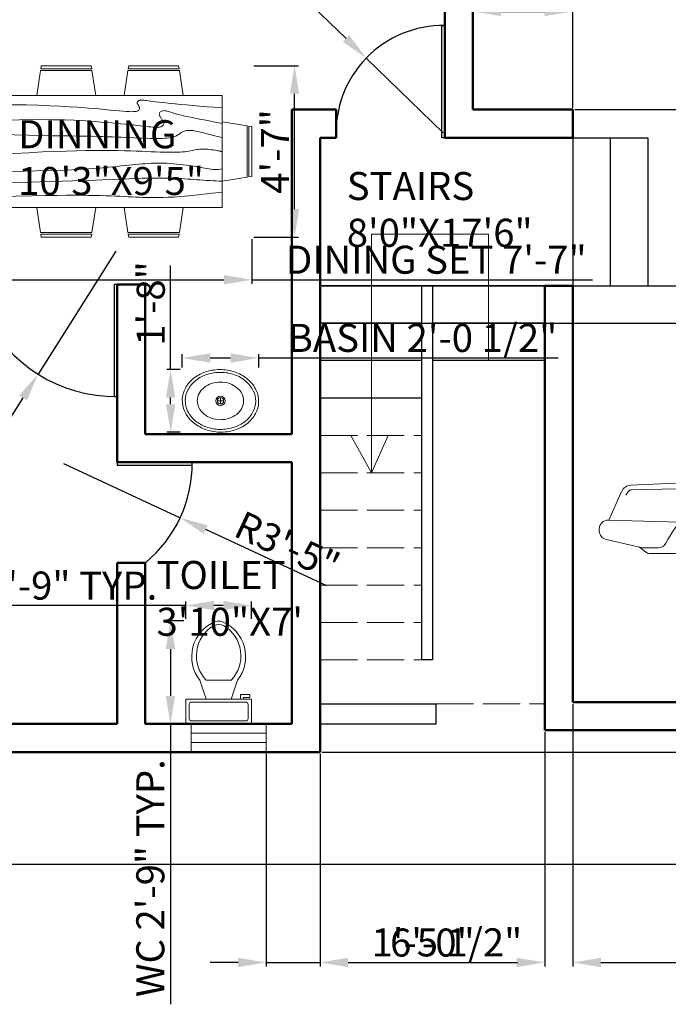
# Model space of a CAD drawing. Units: inches. Extents: x 2059616 to 2060276, y 889994 to 890582.
# Tile 2 of 4: x 2059830 to 2060037, y 890038 to 890354. Entities that reach past the tile are written whole.
import ezdxf

# ---------------------------------------------------------------- set-up
doc = ezdxf.new("R2010")
doc.units = ezdxf.units.IN
doc.linetypes.add('ACAD_ISO02W100', pattern=[15, 12, -3])
for name, color, linetype, lineweight in [('A-ANNO-DIMS', 2, 'Continuous', 18), ('A-ANNO-SYMB', 7, 'Continuous', 18), ('A-AREA-IDEN', 7, 'Continuous', 25), ('A-DOOR', 3, 'Continuous', 25), ('A-FLOR-FIXT', 9, 'Continuous', 18), ('A-FLOR-STRS', 7, 'Continuous', 25), ('A-FLOR-STRS-HIDN', 8, 'ACAD_ISO02W100', 18), ('A-FURN', 8, 'Continuous', 18), ('A-GLAZ', 4, 'Continuous', 18), ('A-SITE-VEHC', 8, 'Continuous', 18), ('A-WALL', 7, 'Continuous', 50), ('C-PROP', 7, 'Continuous', 25)]:
    doc.layers.add(name, color=color, linetype=linetype, lineweight=lineweight)
doc.styles.get("Standard").update_dxf_attribs({"font": 'arial.ttf'})
doc.dimstyles.new('ISO-25', dxfattribs={"dimtxt": 9, "dimasz": 9, "dimexe": 1.25, "dimexo": 0.625, "dimtad": 1, "dimdec": 1, "dimrnd": 9, "dimlunit": 3, "dimtxsty": 'Standard', "dimcen": 2.5, "dimadec": 0, "dimazin": 0, "dimtfac": 1, "dimtdec": 1, "dimtmove": 0, "dimatfit": 3, "dimfxl": 1, "dimarcsym": 0})

# ---------------------------------------------------------------- blocks, each defined once
blk = doc.blocks.new('Car - sedan  side')
for p, q in [((-139.53, 35.99), (-129.64, 47.91)), ((-128.57, 32.64), (-121.22, 48.02)), ((-77.81, 49.34), (-126.58, 49.34)), ((-74.7, 48.02), (-121.22, 48.02)), ((-120.32, 34.67), (-115.67, 48.02)), ((-115.4, 34.67), (-111.74, 48.02)), ((-94.41, 34.67), (-97.73, 48.02)), ((-93.72, 34.67), (-97.04, 48.02)), ((-93.03, 34.67), (-96.34, 48.02)), ((-60.02, 34.65), (-76.07, 48.02)), ((-56.87, 35.13), (-75.48, 48.59)), ((-58.54, 34.93), (-74.99, 48.02)), ((-97.55, 47.3), (-111.94, 47.3)), ((-76.26, 47.3), (-96.16, 47.3)), ((-61.08, 34.66), (-76.26, 47.3)), ((-60.02, 34.65), (-58.54, 34.93)), ((-57.21, 35.38), (-58.54, 34.93)), ((-164.57, 31.6), (-165.48, 30.35)), ((-140.23, 34.67), (-163.88, 33.56)), ((-62.28, 34.67), (-140.23, 34.67)), ((-130.39, 24.63), (-128.57, 32.64)), ((-93.72, 19.62), (-93.72, 34.67)), ((-62.28, 34.67), (-60.02, 34.65)), ((-57.97, 31.61), (-60.02, 34.65)), ((-57.97, 19.62), (-57.97, 31.61)), ((-54.93, 34.4), (-8.75, 29.8)), ((-170.93, 22.32), (-166.81, 31.56)), ((-4.21, 24.18), (-5.42, 27.27)), ((-148.26, 21.7), (-171.11, 22.33)), ((-128.78, 24.63), (-144.79, 24.63)), ((-36.97, 24.38), (-34.94, 24.38)), ((-174, 19.51), (-174, 18.91)), ((-47.2, 19.62), (-125.23, 19.62)), ((-93.72, 12.14), (-93.72, 19.62)), ((-57.97, 12.14), (-57.97, 19.62)), ((0, 19.62), (-24.7, 19.62)), ((-160.12, 13.48), (-171.81, 16.16)), ((-159.22, 12.14), (-161.08, 13.7)), ((-155.01, 13.48), (-160.12, 13.48)), ((-51.4, 9.89), (-49.69, 15.14)), ((-4.23, 13.19), (-20.72, 13.19)), ((-9.5, 13.19), (-14.1, 10.2)), ((-3.22, 13.59), (-1.77, 14.97)), ((-147.03, 11.6), (-157.73, 11.6)), ((-50.67, 12.14), (-123.32, 12.14)), ((-94.21, 9.03), (-94.21, 12.14)), ((-58.39, 9.03), (-58.39, 12.14)), ((-20.36, 11.06), (-24.06, 9.44)), ((-18.83, 10.42), (-19.11, 10.76)), ((-14.68, 10.03), (-18.01, 10.03)), ((-120.62, 9.03), (-125.23, 9.03)), ((-45.76, 9.03), (-120.62, 9.03))]:
    blk.add_line(p, q)
at = {"const_width": 5.49}
for points in [[(-127.8, 11, -1), (-144.3, 11, -1)], [(-26.69, 11, -1), (-43.19, 11, -1)]]:
    blk.add_lwpolyline(points, format="xyb", close=True, dxfattribs=at)
for centre, radius in [((-136.05, 11), 11), ((-34.94, 11), 11), ((-136.05, 11), 5.51), ((-34.94, 11), 5.51)]:
    blk.add_circle(centre, radius)
for centre, radius, start, end in [((-126.58, 45.38), 3.97, 90, 140.3029), ((-77.81, 45.38), 3.97, 54.135, 90), ((-142.58, 38.53), 3.97, 272.6827, 320.3029), ((-54.54, 38.35), 3.97, 234.135, 264.3123), ((-163.72, 30.18), 3.38, 92.6827, 155.9736), ((-163.62, 30.91), 1.17, 91.491, 143.9553), ((-118.51, -1702.12), 1734.79, 86.34698, 91.49105), ((-9.15, 25.82), 4, 21.3107, 84.3123), ((-171.18, 19.51), 2.82, 88.4193, 180), ((-118.09, -2.78), 38.85, 136.3964, 152.9097), ((-144.79, 22.64), 1.98, 90, 136.3964), ((-128.78, 22.64), 1.98, 28.1371, 90), ((-157.14, 7.48), 34.14, 6.5135, 28.1371), ((-36.97, 11), 13.38, 90, 161.9732), ((-34.94, 11), 13.38, 13.5864, 90), ((0.9, 26.18), 5.49, 201.3107, 247.7048), ((-1.92, 19.3), 1.94, 325.3744, 67.7048), ((-171.18, 18.91), 2.82, 180, 257.0905), ((-3.82, 17.12), 2.96, 313.7173, 352.3839), ((2.46, 16.28), 3.37, 145.3744, 172.3839), ((-155.01, 16.1), 2.62, 270, 332.9097), ((-20.72, 14.43), 1.24, 193.5864, 270), ((-4.23, 14.65), 1.46, 270, 313.7173), ((-157.73, 13.93), 2.32, 230.1291, 270), ((-120.62, 11.65), 2.62, 186.5135, 270), ((-52.58, 10.27), 1.24, 270, 341.9732), ((-19.93, 10.09), 1.06, 39.301, 113.7159), ((-18.01, 11.09), 1.06, 219.301, 270), ((-14.68, 11.09), 1.06, 270, 303.047)]:
    blk.add_arc(centre, radius, start, end)
blk = doc.blocks.new('Sink - Oval top')
for p, q in [((-1, 0), (1, 0)), ((0, 1), (0, -1))]:
    blk.add_line(p, q)
for points in [[(-12.23, 0.39, 0.117634), (-11.46, -3.36, 0.104469), (-8.88, -6.8, 0.090016), (-5.08, -9.07, 0.08192), (-0.32, -10.02, 0.08192), (4.49, -9.38, 0.090016), (8.42, -7.36, 0.104469), (11.22, -4.09, 0.117634), (12.23, -0.39, 0.117634), (11.46, 3.36, 0.104469), (8.88, 6.8, 0.090016), (5.08, 9.07, 0.08192), (0.32, 10.02, 0.08192), (-4.49, 9.38, 0.090016), (-8.42, 7.36, 0.104469), (-11.22, 4.09, 0.117634)], [(-11.29, 0.16, 0.118622), (-10.52, -3.25, 0.104678), (-8.07, -6.36, 0.089562), (-4.54, -8.37, 0.081185), (-0.13, -9.15, 0.081185), (4.3, -8.49, 0.089562), (7.89, -6.58, 0.104678), (10.42, -3.55, 0.118622), (11.29, -0.16, 0.118622), (10.52, 3.25, 0.104678), (8.07, 6.36, 0.089562), (4.54, 8.37, 0.081185), (0.13, 9.15, 0.081185), (-4.3, 8.49, 0.089562), (-7.89, 6.58, 0.104678), (-10.42, 3.55, 0.118622)], [(-7.42, 0.08, 0.118283), (-6.91, -2.17, 0.104607), (-5.29, -4.21, 0.089718), (-2.97, -5.53, 0.081436), (-0.07, -6.04, 0.081436), (2.84, -5.59, 0.089718), (5.2, -4.33, 0.104607), (6.86, -2.32, 0.118283), (7.42, -0.08, 0.118283), (6.91, 2.17, 0.104607), (5.29, 4.21, 0.089718), (2.97, 5.53, 0.081436), (0.07, 6.04, 0.081436), (-2.84, 5.59, 0.089718), (-5.2, 4.33, 0.104607), (-6.86, 2.32, 0.118283)]]:
    blk.add_lwpolyline(points, format="xyb", close=True)
for radius in [1.5, 1]:
    blk.add_circle((0, 0), radius)
blk = doc.blocks.new('Toilet - top')
for p, q in [((9.5, -6), (9.5, -2)), ((-10, -8.5), (-8, -8.5)), ((-10, -9.5), (-10, -8.5)), ((-8, -8.5), (-8, -8)), ((-7, -8), (-7, -9.5)), ((-4, -8), (-6, -14)), ((4, -8), (6, -14)), ((-7, -9.5), (-10, -9.5)), ((4, -14), (-4, -14))]:
    blk.add_line(p, q)
blk.add_lwpolyline([(10.5, -8), (10.5, 0), (-10.5, 0), (-10.5, -8)], close=True)
for points in [[(-9.5, -2), (-9.5, -6)], [(8.5, -1), (-8.5, -1)], [(-8.5, -7), (8.5, -7)]]:
    blk.add_lwpolyline(points)
for centre, radius, start, end in [((-8.62, -1.88), 0.884, 81.8699, 188.1301), ((8.62, -1.88), 0.884, 351.8699, 98.1301), ((-8.62, -6.12), 0.884, 171.8699, 278.1301), ((8.62, -6.12), 0.884, 261.8699, 8.1301), ((3.52, -21.58), 12.17, 141.4691, 247.9714), ((4.2, -21.82), 11.33, 136.3677, 238.9468), ((-3.52, -21.58), 12.17, 292.0284, 38.5307), ((-4.2, -21.82), 11.33, 301.053, 43.6321), ((0, -27.88), 4, 245.7318, 294.2682), ((0, -29), 4, 254.8605, 285.1395)]:
    blk.add_arc(centre, radius, start, end)
blk = doc.blocks.new('Dining Set - 36 x 72 in.')
for p, q in [((-22.2343, 26.00059), (-23.4847, 17.99762)), ((-22.2304, 26), (-5.7608, 26)), ((-22, 27.5), (-22.1562, 26.50042)), ((-5.8416, 26.5), (-22.1534, 26.5)), ((-22, 27.5), (-6, 27.5)), ((-5.8437, 26.49966), (-6, 27.5)), ((-4.5152, 17.99762), (-5.7655, 25.99926)), ((5.7657, 26.00059), (4.5153, 17.99762)), ((5.7696, 26), (22.2392, 26)), ((6, 27.5), (5.8438, 26.50042)), ((22.1584, 26.5), (5.8466, 26.5)), ((6, 27.5), (22, 27.5)), ((22.1563, 26.49966), (22, 27.5)), ((23.4848, 17.99762), (22.2345, 25.99926)), ((36, 18), (-36, 18)), ((-36, 18), (-36, -18)), ((36, -18), (36, 18)), ((-44.0006, 8.23428), (-35.9976, 9.48474)), ((44.0006, 8.23428), (35.9976, 9.48474)), ((-45.5, 8), (-44.5004, 8.15617)), ((-45.5, 8), (-45.5, -8)), ((-44.5, -8.15843), (-44.5, 8.15338)), ((-44, 8.23041), (-44, -8.23915)), ((44, 8.23041), (44, -8.23915)), ((44.5, -8.15843), (44.5, 8.15338)), ((45.5, 8), (44.5005, 8.15617)), ((45.5, 8), (45.5, -8)), ((-44.4997, -8.15631), (-45.5, -8)), ((-35.9976, -9.48476), (-43.9993, -8.2345)), ((35.9976, -9.48476), (43.9993, -8.2345)), ((44.4997, -8.15631), (45.5, -8)), ((-36, -18), (36, -18)), ((-22.2343, -26.0006), (-23.4847, -17.99762)), ((-4.5152, -17.99762), (-5.7655, -25.99928)), ((5.7657, -26.0006), (4.5153, -17.99762)), ((23.4848, -17.99762), (22.2345, -25.99928)), ((-22.2304, -26), (-5.7608, -26)), ((-22, -27.5), (-22.1562, -26.50044)), ((-5.8416, -26.5), (-22.1534, -26.5)), ((-22, -27.5), (-6, -27.5)), ((-5.8437, -26.49967), (-6, -27.5)), ((5.7696, -26), (22.2392, -26)), ((6, -27.5), (5.8438, -26.50044)), ((22.1584, -26.5), (5.8466, -26.5)), ((6, -27.5), (22, -27.5)), ((22.1563, -26.49967), (22, -27.5))]:
    blk.add_line(p, q)
for points in [[(-36, 15), (-31.1772, 14.97754), (-26.8079, 14.91406), (-22.8538, 14.81543), (-19.276, 14.6875), (-16.0362, 14.53613), (-13.0957, 14.36718), (-10.4159, 14.18652), (-7.9583, 14), (-5.6904, 13.81315), (-3.6035, 13.63021), (-1.6954, 13.45508), (0.0365, 13.29166), (1.5945, 13.14388), (2.9811, 13.01562), (4.1988, 12.9108), (5.25, 12.83333), (6.1393, 12.78613), (6.8802, 12.76823), (7.4883, 12.77767), (7.9792, 12.8125), (8.3685, 12.87077), (8.6719, 12.95052), (8.9049, 13.0498), (9.0833, 13.16666), (9.2205, 13.29899), (9.3216, 13.44401), (9.3895, 13.59879), (9.4271, 13.76041), (9.4373, 13.92594), (9.4232, 14.09245), (9.3875, 14.257), (9.3333, 14.41666), (9.2638, 14.56917), (9.1836, 14.71484), (9.0975, 14.85465), (9.0104, 14.98958), (8.9272, 15.1206), (8.8529, 15.2487), (8.7922, 15.37483), (8.75, 15.5), (8.7305, 15.62467), (8.7344, 15.74739), (8.7617, 15.86621), (8.8125, 15.97916), (8.8867, 16.08431), (8.9844, 16.17968), (9.1055, 16.26334), (9.25, 16.33333), (9.4189, 16.38802), (9.6172, 16.42708), (9.8506, 16.45052), (10.125, 16.45833), (10.4463, 16.45052), (10.8203, 16.42708), (11.2529, 16.38802), (11.75, 16.33333), (12.3184, 16.26318), (12.9694, 16.17838), (13.7151, 16.07991), (14.5677, 15.96875), (15.5395, 15.84586), (16.6426, 15.71224), (17.8893, 15.56884), (19.2917, 15.41666), (20.859, 15.25667), (22.5879, 15.08984), (24.4721, 14.91715), (26.5052, 14.73958), (28.6809, 14.5581), (30.9929, 14.3737), (33.4347, 14.18733), (36, 14)], [(-36, 10), (-28.9766, 10.14274), (-23.1725, 10.20442), (-18.4241, 10.19775), (-14.5677, 10.13541), (-11.4399, 10.03011), (-8.877, 9.89453), (-6.7154, 9.74137), (-4.7917, 9.58333), (-2.9698, 9.43082), (-1.2246, 9.28515), (0.4415, 9.14534), (2.026, 9.01041), (3.5266, 8.87939), (4.9408, 8.7513), (6.266, 8.62516), (7.5, 8.5), (8.6411, 8.37549), (9.6914, 8.2539), (10.6538, 8.13818), (11.5312, 8.03125), (12.3267, 7.93603), (13.043, 7.85547), (13.6831, 7.79248), (14.25, 7.75), (14.7471, 7.7303), (15.1797, 7.73307), (15.5537, 7.75732), (15.875, 7.80208), (16.1494, 7.86637), (16.3828, 7.94922), (16.5811, 8.04964), (16.75, 8.16666), (16.8944, 8.29915), (17.0143, 8.44531), (17.1089, 8.60319), (17.1771, 8.77083), (17.218, 8.94629), (17.2305, 9.1276), (17.2137, 9.31282), (17.1667, 9.5), (17.0895, 9.6875), (16.987, 9.875), (16.8649, 10.0625), (16.7292, 10.25), (16.5856, 10.4375), (16.4401, 10.625), (16.2985, 10.8125), (16.1667, 11), (16.05, 11.18733), (15.9518, 11.3737), (15.8752, 11.5581), (15.8229, 11.73958), (15.798, 11.91715), (15.8034, 12.08984), (15.842, 12.25667), (15.9167, 12.41666), (16.0295, 12.56836), (16.1784, 12.70833), (16.3605, 12.83268), (16.5729, 12.9375), (16.8127, 13.01888), (17.0768, 13.07291), (17.3625, 13.0957), (17.6667, 13.08333), (17.9894, 13.03312), (18.3418, 12.94726), (18.7382, 12.82918), (19.1927, 12.68229), (19.7195, 12.51001), (20.3327, 12.31575), (21.0465, 12.10294), (21.875, 11.875), (22.8357, 11.63354), (23.959, 11.37304), (25.2786, 11.08618), (26.8282, 10.76562), (28.6414, 10.40405), (30.752, 9.99414), (33.1936, 9.52856), (36, 9)], [(-36, 5.5), (-30.7157, 5.3348), (-26.069, 5.20963), (-21.9946, 5.11767), (-18.4271, 5.05208), (-15.3009, 5.00602), (-12.5508, 4.97265), (-10.1112, 4.94515), (-7.9167, 4.91666), (-5.909, 4.88167), (-4.0586, 4.83984), (-2.3429, 4.79215), (-0.7396, 4.73958), (0.7739, 4.6831), (2.22, 4.6237), (3.6213, 4.56233), (5, 4.5), (6.373, 4.43782), (7.7344, 4.3776), (9.0723, 4.32129), (10.375, 4.27083), (11.6309, 4.22819), (12.8281, 4.19531), (13.9551, 4.17415), (15, 4.16666), (15.954, 4.17448), (16.819, 4.19791), (17.6001, 4.23698), (18.3021, 4.29166), (18.9299, 4.36198), (19.4883, 4.44791), (19.9823, 4.54948), (20.4167, 4.66666), (20.7969, 4.79899), (21.1302, 4.94401), (21.4245, 5.09879), (21.6875, 5.26041), (21.9271, 5.42594), (22.1511, 5.59245), (22.3672, 5.757), (22.5834, 5.91666), (22.8065, 6.06868), (23.0404, 6.21093), (23.2879, 6.34147), (23.5521, 6.45833), (23.8358, 6.55957), (24.142, 6.64323), (24.4735, 6.70735), (24.8334, 6.75), (25.2235, 6.76969), (25.642, 6.76692), (26.0858, 6.74267), (26.5521, 6.69791), (27.0379, 6.63362), (27.5404, 6.55078), (28.0565, 6.45036), (28.5834, 6.33333), (29.1242, 6.19987), (29.7071, 6.04687), (30.3661, 5.87044), (31.1354, 5.66666), (32.0493, 5.43164), (33.142, 5.16146), (34.4475, 4.85221), (36, 4.5)], [(-36, -1), (-30.7915, -0.6591), (-26.0195, -0.38216), (-21.6519, -0.16284), (-17.6563, 0.00521), (-14.0005, 0.12833), (-10.6523, 0.21289), (-7.5796, 0.26522), (-4.75, 0.29166), (-2.134, 0.29793), (0.2878, 0.28711), (2.5317, 0.26163), (4.6146, 0.22396), (6.5529, 0.17651), (8.3633, 0.12174), (10.0623, 0.06209), (11.6667, 0), (13.1899, -0.06201), (14.6341, -0.1211), (15.9982, -0.17432), (17.2813, -0.21875), (18.4823, -0.25147), (19.6003, -0.26953), (20.6343, -0.27002), (21.5834, -0.25), (22.4481, -0.20768), (23.2357, -0.14584), (23.9549, -0.06836), (24.6146, 0.02083), (25.2235, 0.11784), (25.7904, 0.21875), (26.3241, 0.31966), (26.8334, 0.41666), (27.3265, 0.50618), (27.8099, 0.58593), (28.2894, 0.65397), (28.7709, 0.70833), (29.2601, 0.74707), (29.763, 0.76823), (30.2855, 0.76985), (30.8334, 0.75), (31.4088, 0.70784), (31.9994, 0.64713), (32.589, 0.57275), (33.1615, 0.48958), (33.7008, 0.4025), (34.1908, 0.3164), (34.6153, 0.23616), (34.9584, 0.16666), (35.2099, 0.11165), (35.3848, 0.07031), (35.504, 0.04069), (35.5886, 0.02083), (35.6594, 0.00879), (35.7377, 0.0026), (35.8442, 0.00032), (36, 0)], [(-36, -6.5), (-27.1843, -6.31267), (-20.084, -6.1263), (-14.469, -5.9419), (-10.1094, -5.76042), (-6.7752, -5.58285), (-4.2363, -5.41016), (-2.2629, -5.24333), (-0.625, -5.08334), (0.8708, -4.93099), (2.2715, -4.78646), (3.5872, -4.64974), (4.8281, -4.52084), (6.0046, -4.39974), (7.127, -4.28646), (8.2053, -4.18099), (9.25, -4.08334), (10.2705, -3.99382), (11.2734, -3.91407), (12.2647, -3.84603), (13.25, -3.79167), (14.2354, -3.75293), (15.2266, -3.73177), (16.2295, -3.73015), (17.25, -3.75), (18.2912, -3.79248), (19.3451, -3.85547), (20.4009, -3.93604), (21.4479, -4.03125), (22.4754, -4.13819), (23.4727, -4.25391), (24.4289, -4.37549), (25.3334, -4.5), (26.1785, -4.62492), (26.9694, -4.74935), (27.7145, -4.87281), (28.4219, -4.99479), (29.1, -5.11483), (29.7572, -5.23242), (30.4016, -5.34709), (31.0417, -5.45834), (31.6837, -5.56437), (32.3262, -5.65821), (32.9658, -5.73153), (33.599, -5.77604), (34.2224, -5.78345), (34.8327, -5.74545), (35.4264, -5.65373), (36, -5.5)], [(-36, -10), (-26.4022, -9.81299), (-18.4675, -9.62891), (-11.9839, -9.45069), (-6.7396, -9.28125), (-2.5226, -9.12354), (0.8789, -8.98047), (3.6769, -8.85498), (6.0833, -8.75), (8.2767, -8.66765), (10.3021, -8.60677), (12.1712, -8.56543), (13.8958, -8.54167), (15.4876, -8.53353), (16.9583, -8.53907), (18.3197, -8.55632), (19.5834, -8.58334), (20.7616, -8.61841), (21.8685, -8.66081), (22.9188, -8.71004), (23.9271, -8.76563), (24.9081, -8.82707), (25.8763, -8.89388), (26.8465, -8.96558), (27.8334, -9.04167), (28.8474, -9.12118), (29.8828, -9.20117), (30.93, -9.27824), (31.9792, -9.34896), (33.0205, -9.40991), (34.0443, -9.45768), (35.0407, -9.48885), (36, -9.5)], [(-36, -14.5), (-30.0881, -14.33513), (-25.0332, -14.21224), (-20.7312, -14.12647), (-17.0781, -14.07292), (-13.97, -14.04671), (-11.3027, -14.04297), (-8.9724, -14.05681), (-6.875, -14.08334), (-4.9224, -14.11833), (-3.0905, -14.16016), (-1.3709, -14.20785), (0.2448, -14.26042), (1.7647, -14.3169), (3.1973, -14.3763), (4.5507, -14.43767), (5.8333, -14.5), (7.0554, -14.5621), (8.235, -14.62175), (9.3922, -14.67652), (10.5469, -14.72396), (11.7192, -14.76164), (12.929, -14.78711), (14.1965, -14.79794), (15.5417, -14.79167), (16.9933, -14.76424), (18.6152, -14.70508), (20.4804, -14.60197), (22.6615, -14.44271), (25.2312, -14.21509), (28.2624, -13.9069), (31.8277, -13.50594), (36, -13)]]:
    blk.add_lwpolyline(points)
blk = doc.blocks.new('WIN-24IN')
for p, q in [((0, 24), (9, 24)), ((3, 24), (3, 0)), ((6, 24), (6, 0)), ((0, 0), (9, 0))]:
    blk.add_line(p, q)
blk = doc.blocks.new('*D24')
at = {"layer": 'A-ANNO-DIMS', "color": 0, "lineweight": -2, "transparency": 16777216}
for p, q in [((2059882.14, 890160.89), (2059876.56, 890160.89)), ((2059877.81, 890151.89), (2059877.81, 890136.85)), ((2059882.14, 890127.85), (2059876.56, 890127.85)), ((2059877.81, 890127.85), (2059877.81, 890037.93))]:
    blk.add_line(p, q, dxfattribs=at)
at = {"layer": 'A-ANNO-DIMS', "color": 0, "transparency": 16777216}
for points in [[(2059876.31, 890151.89), (2059879.31, 890151.89), (2059877.81, 890160.89)], [(2059876.31, 890136.85), (2059879.31, 890136.85), (2059877.81, 890127.85)]]:
    blk.add_solid(points, dxfattribs=at)
at = {"layer": 'Defpoints', "color": 0, "transparency": 16777216}
for p in [(2059882.76, 890160.89), (2059877.81, 890127.85), (2059882.76, 890127.85)]:
    blk.add_point(p, dxfattribs=at)
at = {"layer": 'A-ANNO-DIMS', "color": 0, "transparency": 16777216, "insert": (2059872.53, 890078.39), "char_height": 9, "attachment_point": 5, "rotation": 90}
blk.add_mtext('WC 2\'-9" TYP.', dxfattribs=at)
blk = doc.blocks.new('*D25')
at = {"layer": 'A-ANNO-DIMS', "color": 0, "lineweight": -2, "transparency": 16777216}
for p, q in [((2059882.76, 890165.85), (2059818.5, 890165.85)), ((2059882.76, 890161.52), (2059882.76, 890167.1)), ((2059894.76, 890165.85), (2059891.76, 890165.85)), ((2059903.76, 890161.52), (2059903.76, 890167.1))]:
    blk.add_line(p, q, dxfattribs=at)
at = {"layer": 'A-ANNO-DIMS', "color": 0, "transparency": 16777216}
for points in [[(2059891.76, 890167.35), (2059891.76, 890164.35), (2059882.76, 890165.85)], [(2059894.76, 890167.35), (2059894.76, 890164.35), (2059903.76, 890165.85)]]:
    blk.add_solid(points, dxfattribs=at)
at = {"layer": 'Defpoints', "color": 0, "transparency": 16777216}
for p in [(2059882.76, 890165.85), (2059882.76, 890160.89), (2059903.76, 890160.89)]:
    blk.add_point(p, dxfattribs=at)
at = {"layer": 'A-ANNO-DIMS', "color": 0, "transparency": 16777216, "insert": (2059846.13, 890171.07), "char_height": 9, "attachment_point": 5}
blk.add_mtext('1\'-9" TYP.', dxfattribs=at)
blk = doc.blocks.new('*D28')
at = {"layer": 'A-ANNO-DIMS', "color": 0, "lineweight": -2, "transparency": 16777216}
for p, q in [((2059881.56, 890242.17), (2059881.56, 890246.48)), ((2059890.56, 890245.23), (2059897.11, 890245.23)), ((2059906.11, 890242.17), (2059906.11, 890246.48)), ((2059906.11, 890245.23), (2060002.08, 890245.23))]:
    blk.add_line(p, q, dxfattribs=at)
at = {"layer": 'A-ANNO-DIMS', "color": 0, "transparency": 16777216}
for points in [[(2059890.56, 890246.73), (2059890.56, 890243.73), (2059881.56, 890245.23)], [(2059897.11, 890246.73), (2059897.11, 890243.73), (2059906.11, 890245.23)]]:
    blk.add_solid(points, dxfattribs=at)
at = {"layer": 'Defpoints', "color": 0, "transparency": 16777216}
for p in [(2059906.11, 890245.23), (2059881.56, 890241.54), (2059906.11, 890241.54)]:
    blk.add_point(p, dxfattribs=at)
at = {"layer": 'A-ANNO-DIMS', "color": 0, "transparency": 16777216, "insert": (2059958.6, 890250.51), "char_height": 9, "attachment_point": 5}
blk.add_mtext('BASIN 2\'-0 1/2"', dxfattribs=at)
blk = doc.blocks.new('*D29')
at = {"layer": 'A-ANNO-DIMS', "color": 0, "lineweight": -2, "transparency": 16777216}
for p, q in [((2059877.88, 890241.54), (2059877.88, 890274.87)), ((2059880.93, 890241.54), (2059876.63, 890241.54)), ((2059877.88, 890230.41), (2059877.88, 890232.54)), ((2059880.93, 890221.41), (2059876.63, 890221.41))]:
    blk.add_line(p, q, dxfattribs=at)
at = {"layer": 'A-ANNO-DIMS', "color": 0, "transparency": 16777216}
for points in [[(2059876.38, 890232.54), (2059879.38, 890232.54), (2059877.88, 890241.54)], [(2059876.38, 890230.41), (2059879.38, 890230.41), (2059877.88, 890221.41)]]:
    blk.add_solid(points, dxfattribs=at)
at = {"layer": 'Defpoints', "color": 0, "transparency": 16777216}
for p in [(2059877.88, 890241.54), (2059881.56, 890241.54), (2059881.56, 890221.41)]:
    blk.add_point(p, dxfattribs=at)
at = {"layer": 'A-ANNO-DIMS', "color": 0, "transparency": 16777216, "insert": (2059872.66, 890262.71), "char_height": 9, "attachment_point": 5, "rotation": 90}
blk.add_mtext('1\'-8"', dxfattribs=at)
blk = doc.blocks.new('*D36')
at = {"layer": 'A-ANNO-DIMS', "color": 0, "lineweight": -2, "transparency": 16777216}
for p, q in [((2059812.93, 890283.34), (2059812.93, 890269.07)), ((2059903.93, 890283.34), (2059903.93, 890269.07)), ((2059821.93, 890270.32), (2059894.93, 890270.32)), ((2059903.93, 890270.32), (2060013.1, 890270.32))]:
    blk.add_line(p, q, dxfattribs=at)
at = {"layer": 'A-ANNO-DIMS', "color": 0, "transparency": 16777216}
for points in [[(2059821.93, 890271.82), (2059821.93, 890268.82), (2059812.93, 890270.32)], [(2059894.93, 890271.82), (2059894.93, 890268.82), (2059903.93, 890270.32)]]:
    blk.add_solid(points, dxfattribs=at)
at = {"layer": 'Defpoints', "color": 0, "transparency": 16777216}
for p in [(2059812.93, 890283.97), (2059903.93, 890283.97), (2059903.93, 890270.32)]:
    blk.add_point(p, dxfattribs=at)
at = {"layer": 'A-ANNO-DIMS', "color": 0, "transparency": 16777216, "insert": (2059963.02, 890275.59), "char_height": 9, "attachment_point": 5}
blk.add_mtext('DINING SET 7\'-7"', dxfattribs=at)
blk = doc.blocks.new('*D37')
at = {"layer": 'A-ANNO-DIMS', "color": 0, "lineweight": -2, "transparency": 16777216}
for p, q in [((2059904.56, 890338.97), (2059918.83, 890338.97)), ((2059917.58, 890292.97), (2059917.58, 890329.97)), ((2059904.56, 890283.97), (2059918.83, 890283.97))]:
    blk.add_line(p, q, dxfattribs=at)
at = {"layer": 'A-ANNO-DIMS', "color": 0, "transparency": 16777216}
for points in [[(2059916.08, 890329.97), (2059919.08, 890329.97), (2059917.58, 890338.97)], [(2059916.08, 890292.97), (2059919.08, 890292.97), (2059917.58, 890283.97)]]:
    blk.add_solid(points, dxfattribs=at)
at = {"layer": 'Defpoints', "color": 0, "transparency": 16777216}
for p in [(2059903.93, 890338.97), (2059917.58, 890338.97), (2059903.93, 890283.97)]:
    blk.add_point(p, dxfattribs=at)
at = {"layer": 'A-ANNO-DIMS', "color": 0, "transparency": 16777216, "insert": (2059912.46, 890311.47), "char_height": 9, "attachment_point": 5, "rotation": 90}
blk.add_mtext('4\'-7"', dxfattribs=at)
blk = doc.blocks.new('*D39')
at = {"layer": 'A-ANNO-DIMS', "color": 0, "lineweight": -2, "transparency": 16777216}
for p, q in [((2060202.39, 890497.85), (2060275.51, 890497.85)), ((2060274.26, 890127.85), (2060274.26, 890488.85)), ((2059926.39, 890118.85), (2060275.51, 890118.85))]:
    blk.add_line(p, q, dxfattribs=at)
at = {"layer": 'A-ANNO-DIMS', "color": 0, "transparency": 16777216}
for points in [[(2060272.76, 890488.85), (2060275.76, 890488.85), (2060274.26, 890497.85)], [(2060272.76, 890127.85), (2060275.76, 890127.85), (2060274.26, 890118.85)]]:
    blk.add_solid(points, dxfattribs=at)
at = {"layer": 'Defpoints', "color": 0, "transparency": 16777216}
for p in [(2060201.76, 890497.85), (2060274.26, 890497.85), (2059925.76, 890118.85)]:
    blk.add_point(p, dxfattribs=at)
at = {"layer": 'A-ANNO-DIMS', "color": 0, "transparency": 16777216, "insert": (2060269.04, 890308.35), "char_height": 9, "attachment_point": 5, "rotation": 90}
blk.add_mtext('31\'-7"', dxfattribs=at)
blk = doc.blocks.new('*D52')
at = {"layer": 'A-ANNO-DIMS', "color": 0, "lineweight": -2, "transparency": 16777216}
for p, q in [((2059908.5, 890118.22), (2059908.5, 890050.1)), ((2059925.76, 890118.22), (2059925.76, 890050.1)), ((2059899.5, 890051.35), (2059890.5, 890051.35)), ((2059908.5, 890051.35), (2059925.76, 890051.35)), ((2059934.76, 890051.35), (2059989.06, 890051.35))]:
    blk.add_line(p, q, dxfattribs=at)
at = {"layer": 'A-ANNO-DIMS', "color": 0, "transparency": 16777216}
for points in [[(2059899.5, 890052.85), (2059899.5, 890049.85), (2059908.5, 890051.35)], [(2059934.76, 890052.85), (2059934.76, 890049.85), (2059925.76, 890051.35)]]:
    blk.add_solid(points, dxfattribs=at)
at = {"layer": 'Defpoints', "color": 0, "transparency": 16777216}
for p in [(2059908.5, 890118.85), (2059925.76, 890118.85), (2059925.76, 890051.35)]:
    blk.add_point(p, dxfattribs=at)
at = {"layer": 'A-ANNO-DIMS', "color": 0, "transparency": 16777216, "insert": (2059966.41, 890056.62), "char_height": 9, "attachment_point": 5}
blk.add_mtext('1\'-5 1/2"', dxfattribs=at)
blk = doc.blocks.new('*D54')
at = {"layer": 'A-ANNO-DIMS', "color": 0, "lineweight": -2, "transparency": 16777216}
for p, q in [((2059974.76, 890325.51), (2059974.76, 890357.64)), ((2060006.76, 890325.51), (2060006.76, 890357.64)), ((2059983.76, 890356.39), (2059997.76, 890356.39))]:
    blk.add_line(p, q, dxfattribs=at)
at = {"layer": 'A-ANNO-DIMS', "color": 0, "transparency": 16777216}
for points in [[(2059983.76, 890357.89), (2059983.76, 890354.89), (2059974.76, 890356.39)], [(2059997.76, 890357.89), (2059997.76, 890354.89), (2060006.76, 890356.39)]]:
    blk.add_solid(points, dxfattribs=at)
at = {"layer": 'Defpoints', "color": 0, "transparency": 16777216}
for p in [(2060006.76, 890356.39), (2059974.76, 890324.89), (2060006.76, 890324.89)]:
    blk.add_point(p, dxfattribs=at)
at = {"layer": 'A-ANNO-DIMS', "color": 0, "transparency": 16777216, "insert": (2059990.76, 890361.61), "char_height": 9, "attachment_point": 5}
blk.add_mtext('2\'-8"', dxfattribs=at)
blk = doc.blocks.new('*D55')
at = {"layer": 'A-ANNO-DIMS', "color": 0, "lineweight": -2, "transparency": 16777216}
for p, q in [((2060007.39, 890324.89), (2060275.51, 890324.89)), ((2060274.26, 890315.89), (2060274.26, 890143.85)), ((2060007.39, 890134.85), (2060275.51, 890134.85))]:
    blk.add_line(p, q, dxfattribs=at)
at = {"layer": 'A-ANNO-DIMS', "color": 0, "transparency": 16777216}
for points in [[(2060272.76, 890315.89), (2060275.76, 890315.89), (2060274.26, 890324.89)], [(2060272.76, 890143.85), (2060275.76, 890143.85), (2060274.26, 890134.85)]]:
    blk.add_solid(points, dxfattribs=at)
at = {"layer": 'Defpoints', "color": 0, "transparency": 16777216}
for p in [(2060006.76, 890324.89), (2060006.76, 890134.85), (2060274.26, 890134.85)]:
    blk.add_point(p, dxfattribs=at)
at = {"layer": 'A-ANNO-DIMS', "color": 0, "transparency": 16777216, "insert": (2060269.04, 890229.87), "char_height": 9, "attachment_point": 5, "rotation": 90}
blk.add_mtext('15\'-10"', dxfattribs=at)
blk = doc.blocks.new('*D56')
at = {"layer": 'A-ANNO-DIMS', "color": 0, "lineweight": -2, "transparency": 16777216}
for p, q in [((2060006.76, 890134.22), (2060006.76, 890050.1)), ((2060192.76, 890134.22), (2060192.76, 890050.1)), ((2060015.76, 890051.35), (2060183.76, 890051.35))]:
    blk.add_line(p, q, dxfattribs=at)
at = {"layer": 'A-ANNO-DIMS', "color": 0, "transparency": 16777216}
for points in [[(2060015.76, 890052.85), (2060015.76, 890049.85), (2060006.76, 890051.35)], [(2060183.76, 890052.85), (2060183.76, 890049.85), (2060192.76, 890051.35)]]:
    blk.add_solid(points, dxfattribs=at)
at = {"layer": 'Defpoints', "color": 0, "transparency": 16777216}
for p in [(2060006.76, 890134.85), (2060192.76, 890134.85), (2060192.76, 890051.35)]:
    blk.add_point(p, dxfattribs=at)
at = {"layer": 'A-ANNO-DIMS', "color": 0, "transparency": 16777216, "insert": (2060099.76, 890056.57), "char_height": 9, "attachment_point": 5}
blk.add_mtext('15\'-6"', dxfattribs=at)
blk = doc.blocks.new('*D57')
at = {"layer": 'A-ANNO-DIMS', "color": 0, "lineweight": -2, "transparency": 16777216}
for p, q in [((2059997.76, 890125.22), (2059997.76, 890050.1)), ((2059925.76, 890118.22), (2059925.76, 890050.1)), ((2059934.76, 890051.35), (2059988.76, 890051.35))]:
    blk.add_line(p, q, dxfattribs=at)
at = {"layer": 'A-ANNO-DIMS', "color": 0, "transparency": 16777216}
for points in [[(2059934.76, 890052.85), (2059934.76, 890049.85), (2059925.76, 890051.35)], [(2059988.76, 890052.85), (2059988.76, 890049.85), (2059997.76, 890051.35)]]:
    blk.add_solid(points, dxfattribs=at)
at = {"layer": 'Defpoints', "color": 0, "transparency": 16777216}
for p in [(2059997.76, 890125.85), (2059925.76, 890118.85), (2059997.76, 890051.35)]:
    blk.add_point(p, dxfattribs=at)
at = {"layer": 'A-ANNO-DIMS', "color": 0, "transparency": 16777216, "insert": (2059961.76, 890056.57), "char_height": 9, "attachment_point": 5}
blk.add_mtext('6\'-0"', dxfattribs=at)
blk = doc.blocks.new('*D59')
at = {"layer": 'A-ANNO-DIMS', "color": 0, "lineweight": -2, "transparency": 16777216}
for p, q in [((2060274.26, 890277.39), (2060274.26, 890310.71)), ((2059926.39, 890268.39), (2060275.51, 890268.39)), ((2060274.26, 890256.39), (2060274.26, 890268.39)), ((2059926.39, 890256.39), (2060275.51, 890256.39)), ((2060274.26, 890247.39), (2060274.26, 890238.39))]:
    blk.add_line(p, q, dxfattribs=at)
at = {"layer": 'A-ANNO-DIMS', "color": 0, "transparency": 16777216}
for points in [[(2060272.76, 890277.39), (2060275.76, 890277.39), (2060274.26, 890268.39)], [(2060272.76, 890247.39), (2060275.76, 890247.39), (2060274.26, 890256.39)]]:
    blk.add_solid(points, dxfattribs=at)
at = {"layer": 'Defpoints', "color": 0, "transparency": 16777216}
for p in [(2059925.76, 890268.39), (2060274.26, 890268.39), (2059925.76, 890256.39)]:
    blk.add_point(p, dxfattribs=at)
at = {"layer": 'A-ANNO-DIMS', "color": 0, "transparency": 16777216, "insert": (2060269.04, 890298.55), "char_height": 9, "attachment_point": 5, "rotation": 90}
blk.add_mtext('1\'-0"', dxfattribs=at)
blk = doc.blocks.new('*D60')
at = {"layer": 'A-ANNO-DIMS', "color": 0, "lineweight": -2, "transparency": 16777216}
for p, q in [((2059860.26, 890279.49), (2059835.38, 890240.04)), ((2059792.83, 890172.58), (2059830.58, 890232.42))]:
    blk.add_line(p, q, dxfattribs=at)
at = {"layer": 'A-ANNO-DIMS', "color": 0, "transparency": 16777216}
blk.add_solid([(2059829.31, 890233.22), (2059831.85, 890231.62), (2059835.38, 890240.04)], dxfattribs=at)
at = {"layer": 'Defpoints', "color": 0, "transparency": 16777216}
for p in [(2059860.26, 890279.49), (2059835.38, 890240.04)]:
    blk.add_point(p, dxfattribs=at)
at = {"layer": 'A-ANNO-DIMS', "color": 0, "transparency": 16777216, "insert": (2059804.84, 890201.51), "char_height": 9, "attachment_point": 5, "rotation": 57.7581}
blk.add_mtext('R3\'-10 1/2"', dxfattribs=at)
blk = doc.blocks.new('*D61')
at = {"layer": 'A-ANNO-DIMS', "color": 0, "lineweight": -2, "transparency": 16777216}
for p, q in [((2059843.58, 890211.35), (2059880.93, 890193.99)), ((2059927.9, 890172.18), (2059889.1, 890190.2))]:
    blk.add_line(p, q, dxfattribs=at)
at = {"layer": 'A-ANNO-DIMS', "color": 0, "transparency": 16777216}
blk.add_solid([(2059889.73, 890191.56), (2059888.46, 890188.84), (2059880.93, 890193.99)], dxfattribs=at)
at = {"layer": 'Defpoints', "color": 0, "transparency": 16777216}
for p in [(2059843.58, 890211.35), (2059880.93, 890193.99)]:
    blk.add_point(p, dxfattribs=at)
at = {"layer": 'A-ANNO-DIMS', "color": 0, "transparency": 16777216, "insert": (2059914.78, 890184.03), "char_height": 9, "attachment_point": 5, "rotation": 335.0861}
blk.add_mtext('R3\'-5"', dxfattribs=at)
blk = doc.blocks.new('*D63')
at = {"layer": 'A-ANNO-DIMS', "color": 0, "lineweight": -2, "transparency": 16777216}
for p, q in [((2059883.25, 890396.89), (2059934.09, 890347.68)), ((2059965.26, 890317.5), (2059940.56, 890341.42))]:
    blk.add_line(p, q, dxfattribs=at)
at = {"layer": 'A-ANNO-DIMS', "color": 0, "transparency": 16777216}
blk.add_solid([(2059935.13, 890348.76), (2059933.05, 890346.61), (2059940.56, 890341.42)], dxfattribs=at)
at = {"layer": 'Defpoints', "color": 0, "transparency": 16777216}
for p in [(2059940.56, 890341.42), (2059965.26, 890317.5)]:
    blk.add_point(p, dxfattribs=at)
at = {"layer": 'A-ANNO-DIMS', "color": 0, "transparency": 16777216, "insert": (2059909.11, 890379.21), "char_height": 9, "attachment_point": 5, "rotation": 315.9294}
blk.add_mtext('R2\'-10 1/2"', dxfattribs=at)

msp = doc.modelspace()

# ---------------------------------------------------------------- linework, layer by layer
at = {"layer": 'A-ANNO-SYMB'}
for p, q in [((2059979.76, 890284.98), (2059942.2, 890284.98)), ((2059942.2, 890284.98), (2059942.2, 890208.39)), ((2059979.76, 890244.39), (2059979.76, 890284.98)), ((2059942.2, 890208.39), (2059935.65, 890220.39)), ((2059942.2, 890208.39), (2059947.58, 890220.39))]:
    msp.add_line(p, q, dxfattribs=at)
at = {"layer": 'A-DOOR'}
for p, q in [((2059964.76, 890315.89), (2059964.76, 890351.89)), ((2059964.76, 890351.89), (2059965.76, 890351.89)), ((2059965.76, 890315.89), (2059964.76, 890315.89)), ((2059860.76, 890268.85), (2059859.76, 890268.85)), ((2059859.76, 890268.85), (2059859.76, 890232.85)), ((2059859.76, 890232.85), (2059860.76, 890232.85)), ((2059860.76, 890211.85), (2059860.76, 890210.85)), ((2059884.76, 890210.85), (2059884.76, 890211.85)), ((2059860.76, 890210.85), (2059884.76, 890210.85))]:
    msp.add_line(p, q, dxfattribs=at)
for centre, radius, start, end in [((2059965.26, 890317.5), 34.39, 89.1669, 182.6899), ((2059860.26, 890279.49), 46.64, 204.9024, 270.6142), ((2059843.58, 890211.35), 41.19, 309.4763, 0.6955)]:
    msp.add_arc(centre, radius, start, end, dxfattribs=at)
at = {"layer": 'A-FLOR-STRS'}
for p, q in [((2060006.76, 890315.89), (2060006.76, 890268.39)), ((2060006.76, 890315.89), (2060030.76, 890315.89)), ((2060018.76, 890315.89), (2060018.76, 890268.39)), ((2060030.76, 890315.89), (2060030.76, 890268.39)), ((2059997.76, 890268.39), (2059925.76, 890268.39)), ((2060006.76, 890268.39), (2060030.76, 890268.39)), ((2059958.36, 890256.39), (2059925.76, 890256.39)), ((2059997.76, 890256.39), (2059961.76, 890256.39)), ((2059958.36, 890244.39), (2059925.76, 890244.39)), ((2059997.76, 890244.39), (2059961.76, 890244.39)), ((2059958.36, 890232.39), (2059925.76, 890232.39)), ((2059925.76, 890134.31), (2059962.9, 890134.31)), ((2059962.9, 890134.31), (2059962.9, 890127.78)), ((2059962.9, 890127.78), (2059925.76, 890127.78))]:
    msp.add_line(p, q, dxfattribs=at)
msp.add_lwpolyline([(2059958.36, 890268.39), (2059961.76, 890268.39), (2059961.76, 890148.39), (2059958.36, 890148.39)], close=True, dxfattribs=at)
at = {"layer": 'A-FLOR-STRS-HIDN'}
for p, q in [((2059925.76, 890220.39), (2059958.36, 890220.39)), ((2059925.76, 890208.39), (2059958.36, 890208.39)), ((2059925.76, 890196.39), (2059958.36, 890196.39)), ((2059925.76, 890184.39), (2059958.36, 890184.39)), ((2059925.76, 890172.39), (2059958.36, 890172.39)), ((2059925.76, 890160.39), (2059958.36, 890160.39)), ((2059925.76, 890148.39), (2059961.76, 890148.39)), ((2059962.9, 890134.31), (2059997.76, 890134.31))]:
    msp.add_line(p, q, dxfattribs=at)
at = {"layer": 'A-WALL'}
for p, q in [((2059965.76, 890488.85), (2059965.76, 890315.89)), ((2059974.76, 890488.85), (2059974.76, 890324.89)), ((2059916.76, 890324.89), (2059916.76, 890220.85)), ((2059925.76, 890324.89), (2059916.76, 890324.89)), ((2059925.76, 890324.89), (2059930.91, 890324.89)), ((2059930.91, 890324.89), (2059930.91, 890315.89)), ((2060006.76, 890324.89), (2059974.76, 890324.89)), ((2060006.76, 890324.89), (2060006.76, 890315.89)), ((2059925.76, 890315.89), (2059925.76, 890127.85)), ((2059930.91, 890315.89), (2059925.76, 890315.89)), ((2060006.76, 890315.89), (2059965.76, 890315.89)), ((2059860.76, 890268.85), (2059860.76, 890211.85)), ((2059860.76, 890268.85), (2059869.76, 890268.85)), ((2059869.76, 890268.85), (2059869.76, 890220.85)), ((2059997.76, 890268.39), (2059997.76, 890125.85)), ((2059997.76, 890268.39), (2060006.76, 890268.39)), ((2060006.76, 890268.39), (2060006.76, 890134.85)), ((2059869.76, 890220.85), (2059916.76, 890220.85)), ((2059869.76, 890211.85), (2059860.76, 890211.85)), ((2059869.76, 890211.85), (2059916.76, 890211.85)), ((2059916.76, 890211.85), (2059916.76, 890127.85)), ((2059869.76, 890179.55), (2059860.76, 890179.55)), ((2059860.76, 890179.55), (2059860.76, 890127.85)), ((2059869.76, 890179.55), (2059869.76, 890127.85)), ((2060192.76, 890134.85), (2060006.76, 890134.85)), ((2059716.76, 890127.85), (2059860.76, 890127.85)), ((2059869.76, 890127.85), (2059916.76, 890127.85)), ((2059925.76, 890127.85), (2059925.76, 890118.85)), ((2060192.76, 890125.85), (2059997.76, 890125.85)), ((2059707.76, 890118.85), (2059925.76, 890118.85))]:
    msp.add_line(p, q, dxfattribs=at)
at = {"layer": 'C-PROP'}
msp.add_line((2059666.76, 890082.85), (2060242.76, 890082.85), dxfattribs=at)

# ---------------------------------------------------------------- block references
at = {"layer": 'A-FLOR-FIXT'}
msp.add_blockref('Sink - Oval top', (2059893.84, 890231.48), dxfattribs=at)
at = {"layer": 'A-FLOR-FIXT', "rotation": 180}
msp.add_blockref('Toilet - top', (2059893.26, 890127.85), dxfattribs=at)
at = {"layer": 'A-FURN'}
msp.add_blockref('Dining Set - 36 x 72 in.', (2059858.43, 890311.47), dxfattribs=at)
at = {"layer": 'A-GLAZ', "rotation": 89.9999999974416}
msp.add_blockref('WIN-24IN', (2059908.5, 890118.85), dxfattribs=at)
at = {"layer": 'A-SITE-VEHC'}
msp.add_blockref('Car - sedan  side', (2060189.23, 890170.88), dxfattribs=at)

# ---------------------------------------------------------------- texts
at = {"layer": 'A-AREA-IDEN', "char_height": 9, "attachment_point": 1}
for s, insert in [('DINNING\\P10\'3"X9\'5"', (2059828.99, 890321.5)), ('STAIRS\\P8\'0"X17\'6"', (2059934.32, 890304.89)), ('TOILET\\P3\'10"X7\'', (2059873.35, 890180.13))]:
    msp.add_mtext_dynamic_manual_height_columns(s, width=69.4215, gutter_width=12.5, heights=[0], dxfattribs=dict(at, insert=insert))

# ---------------------------------------------------------------- dimensions: what is measured, and where the dimension line sits
at = {"layer": 'A-ANNO-DIMS'}
for base, p1, p2, picture, middle in [((2060274.26, 890497.85), (2059925.76, 890118.85), (2060201.76, 890497.85), '*D39', (2060269.04, 890308.35)), ((2059917.58, 890338.97), (2059903.93, 890283.97), (2059903.93, 890338.97), '*D37', (2059912.46, 890311.47)), ((2060274.26, 890134.85), (2060006.76, 890324.89), (2060006.76, 890134.85), '*D55', (2060269.04, 890229.87)), ((2060274.26, 890268.39), (2059925.76, 890256.39), (2059925.76, 890268.39), '*D59', (2060269.04, 890298.55)), ((2059877.88, 890241.54), (2059881.56, 890221.41), (2059881.56, 890241.54), '*D29', (2059872.66, 890262.71))]:
    dim = msp.add_linear_dim(base=base, p1=p1, p2=p2, angle=90, dimstyle='ISO-25', override={"dimdec": 1, "dimlfac": 1, "dimrnd": 0, "dimzin": 1, "dimdsep": 46, "dimlunit": 4, "dimfrac": 2}, dxfattribs=at)
    dim.commit()
    dim.dimension.update_dxf_attribs({"geometry": picture, "text_midpoint": middle})
for center, mpoint, picture, middle in [((2059965.26, 890317.5), (2059940.56, 890341.42), '*D63', (2059909.11, 890379.21)), ((2059860.26, 890279.49), (2059835.38, 890240.04), '*D60', (2059804.84, 890201.51)), ((2059843.58, 890211.35), (2059880.93, 890193.99), '*D61', (2059914.78, 890184.03))]:
    dim = msp.add_radius_dim(center=center, mpoint=mpoint, dimstyle='ISO-25', override={"dimdec": 1, "dimlfac": 1, "dimrnd": 0, "dimzin": 1, "dimdsep": 46, "dimlunit": 4, "dimfrac": 2}, dxfattribs=at)
    dim.commit()
    dim.dimension.update_dxf_attribs({"geometry": picture, "text_midpoint": middle})
for base, p1, p2, picture, middle in [((2060006.76, 890356.39), (2059974.76, 890324.89), (2060006.76, 890324.89), '*D54', (2059990.76, 890361.61)), ((2060192.76, 890051.35), (2060006.76, 890134.85), (2060192.76, 890134.85), '*D56', (2060099.76, 890056.57)), ((2059997.76, 890051.35), (2059925.76, 890118.85), (2059997.76, 890125.85), '*D57', (2059961.76, 890056.57)), ((2059925.76, 890051.35), (2059908.5, 890118.85), (2059925.76, 890118.85), '*D52', (2059966.41, 890056.62))]:
    dim = msp.add_linear_dim(base=base, p1=p1, p2=p2, dimstyle='ISO-25', override={"dimdec": 1, "dimlfac": 1, "dimrnd": 0, "dimzin": 1, "dimdsep": 46, "dimlunit": 4, "dimfrac": 2}, dxfattribs=at)
    dim.commit()
    dim.dimension.update_dxf_attribs({"geometry": picture, "text_midpoint": middle})
for base, p1, p2, text, picture, middle in [((2059903.93, 890270.32), (2059812.93, 890283.97), (2059903.93, 890283.97), 'DINING SET <>', '*D36', (2059963.02, 890275.59)), ((2059906.1109, 890245.2272), (2059881.56, 890241.5445), (2059906.1109, 890241.5445), 'BASIN <>', '*D28', (2059958.5964, 890250.5056))]:
    dim = msp.add_linear_dim(base=base, p1=p1, p2=p2, text=text, dimstyle='ISO-25', override={"dimdec": 1, "dimlfac": 1, "dimrnd": 0, "dimzin": 1, "dimdsep": 46, "dimlunit": 4, "dimfrac": 2}, dxfattribs=at)
    dim.commit()
    dim.dimension.update_dxf_attribs({"geometry": picture, "text_midpoint": middle})
for base, p1, p2, angle, text, picture, middle in [((2059882.76, 890165.85), (2059903.76, 890160.89), (2059882.76, 890160.89), 180, '<> TYP.', '*D25', (2059846.13, 890171.07)), ((2059877.81, 890127.85), (2059882.76, 890160.89), (2059882.76, 890127.85), 270, 'WC <> TYP.', '*D24', (2059872.53, 890078.39))]:
    dim = msp.add_linear_dim(base=base, p1=p1, p2=p2, angle=angle, text=text, dimstyle='ISO-25', override={"dimdec": 1, "dimlfac": 1, "dimrnd": 0, "dimzin": 1, "dimdsep": 46, "dimlunit": 4, "dimfrac": 2}, dxfattribs=at)
    dim.commit()
    dim.dimension.update_dxf_attribs({"geometry": picture, "text_midpoint": middle})

doc.saveas('drawing.dxf')
